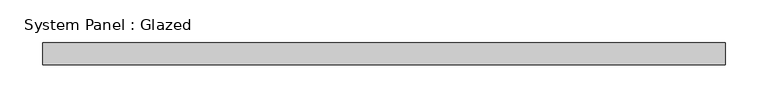
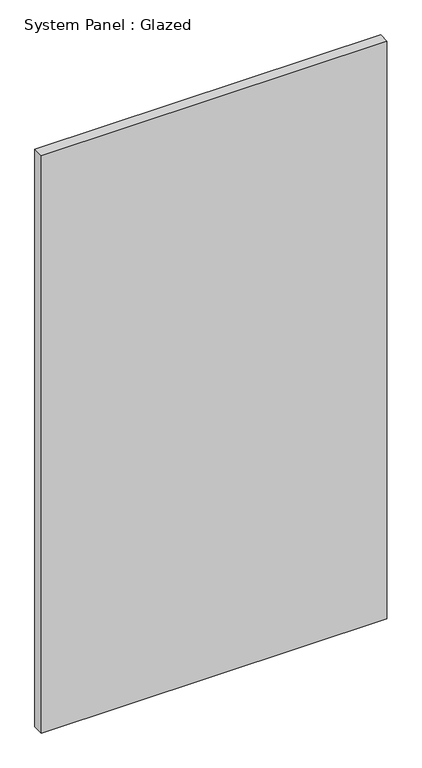
"""IFC4 building model written with IfcOpenShell, lengths in millimetres: plate geometry, System Panel : Glazed."""

from ifc_helpers import new_model, si_unit, origin, origin_with_axes, place, context, project, spatial, polyline, outline, extrude, source, transform, mapped, element, save


def system_panel_glazed_53576031(model_context):
    return source(origin(), model_context, "Body", "SweptSolid", [
        extrude(outline(polyline([(396.875, 19.05), (-396.875, 19.05), (-396.875, 44.45), (396.875, 44.45), (396.875, 19.05)])), origin_with_axes(), (0.0, 0.0, 1.0), 1401.6649662),
    ])


if __name__ == "__main__":
    model = new_model("IFC4")
    model_context = context("Model", 3, world=origin())
    ifc_project = project(units=[si_unit("LENGTHUNIT", "METRE", prefix="MILLI")], contexts=[model_context])
    site = spatial("IfcSite", under=ifc_project)
    building = spatial("IfcBuilding", under=site)
    placement = place(None, origin())
    system_panel_glazed_shape = system_panel_glazed_53576031(model_context)
    element("IfcPlate", 1, ObjectType="System Panel : Glazed", at=placement, inside=building, context=model_context, shape_type="MappedRepresentation", body=[
        mapped(system_panel_glazed_shape, transform((0.0, 0.0, 0.0), x_axis=(1.0, 0.0, 0.0), y_axis=(0.0, 1.0, 0.0), z_axis=(0.0, 0.0, 1.0))),
    ])
    save(model, "model.ifc")

# Revit data of these elements
# Type "System Panel : Glazed"
#   Construction Type Id = "GSP4R"
#   Analytic Construction = "1/8 in Pilkington single glazing"
#   Visual Light Transmittance = 0.9
#   Solar Heat Gain Coefficient = 0.86
#   Heat Transfer Coefficient (U) = 1.18115 BTU/(h·ft²·°F)
#   Define Thermal Properties by = 1
# Element 1 (IfcPlate, "System Panel : Glazed")
#   Materials on its faces: "Glass"
# Materials
#   "Glass": class "Glass", colour RGB 0 128 192, transparency 0.75, Description = "Soda Lime Glass", Cost = 0
